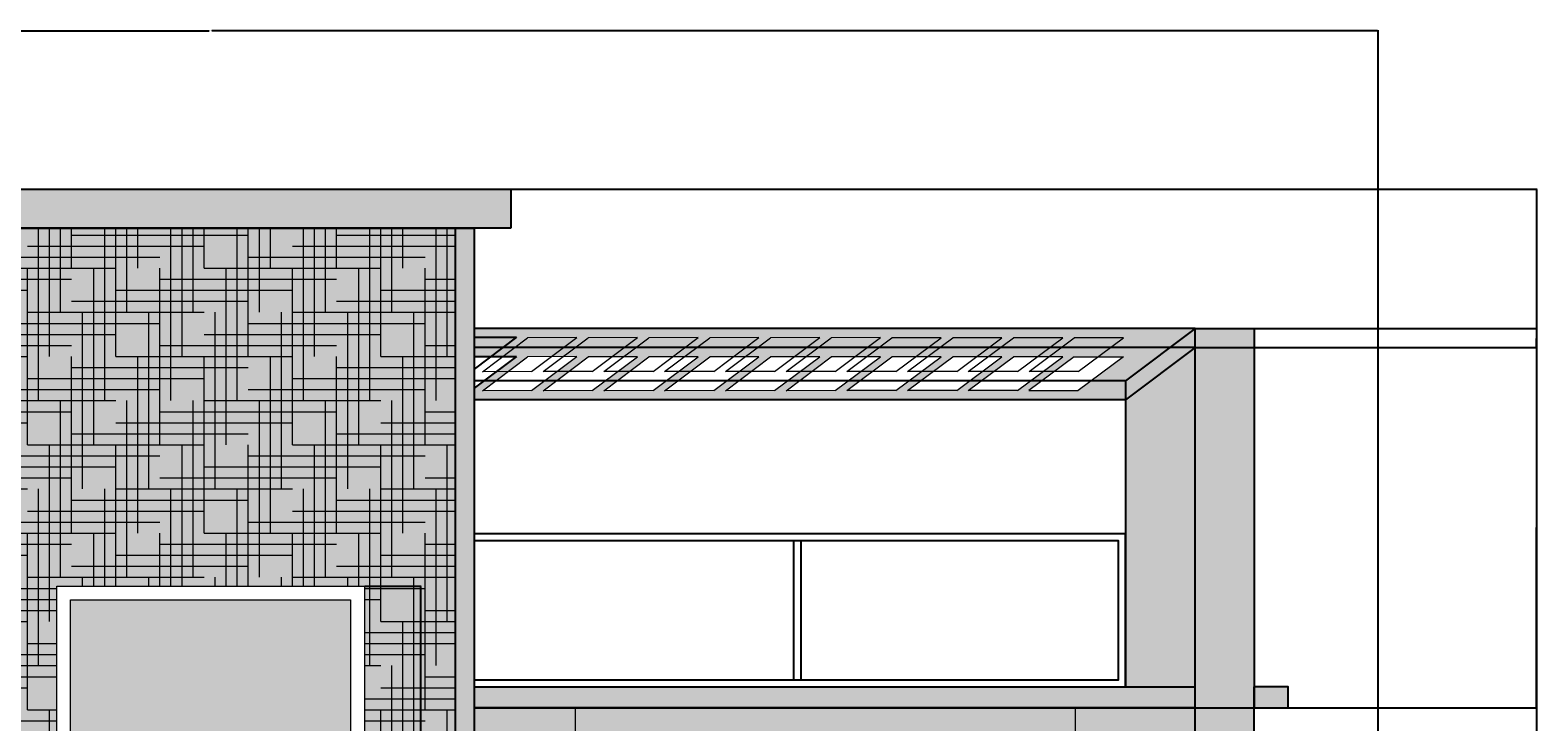
# Model space of a CAD drawing. Units: inches. Extents: x 3024 to 4744, y 1110 to 2100.
# Tile 27 of 29: x 3354 to 3787, y 1902 to 2100. Entities that reach past the tile are written whole.
import ezdxf

# ---------------------------------------------------------------- set-up
doc = ezdxf.new("R2010")
doc.units = ezdxf.units.IN
for name, color, linetype, lineweight in [('A-ANNO-DIMS', 2, 'Continuous', 18), ('A-ELEV', 7, 'Continuous', 25), ('A-ELEV-PATT', 252, 'Continuous', 13), ('A-GLAZ', 4, 'Continuous', 18), ('A-ROOF', 3, 'Continuous', 18)]:
    doc.layers.add(name, color=color, linetype=linetype, lineweight=lineweight)
doc.styles.get("Standard").update_dxf_attribs({"font": 'arial.ttf'})
doc.dimstyles.get("Standard").update_dxf_attribs({"dimtxt": 0.18, "dimasz": 0.18, "dimexe": 0.18, "dimexo": 0.0625, "dimgap": 0.09, "dimtad": 0, "dimtih": 1, "dimtoh": 1, "dimdec": 1, "dimzin": 0, "dimdsep": 46, "dimlunit": 3, "dimtxsty": 'Standard', "dimcen": 0.09, "dimadec": 0, "dimazin": 0, "dimtfac": 1, "dimtdec": 1, "dimtofl": 0, "dimtmove": 0, "dimatfit": 3, "dimfxl": 1, "dimtolj": 1, "dimtzin": 0, "dimarcsym": 0})

# ---------------------------------------------------------------- blocks, each defined once
blk = doc.blocks.new('WIN-BALCONY-A')
for p, q in [((3169.4, 1897.49), (3148.97, 1897.49)), ((3169.4, 1897.49), (3148.97, 1897.49)), ((3169.4, 1897.49), (3292.61, 1897.49)), ((3169.4, 1897.49), (3292.61, 1897.49)), ((3169.4, 1795.04), (3148.97, 1795.04)), ((3169.4, 1795.04), (3148.97, 1795.04)), ((3169.4, 1795.04), (3292.61, 1795.04)), ((3169.4, 1795.04), (3292.61, 1795.04))]:
    blk.add_line(p, q)
for points in [[(3148.97, 1897.49), (3148.97, 1905.61), (3292.61, 1905.61), (3292.61, 1897.49)], [(3148.97, 1897.49), (3148.97, 1905.61), (3292.61, 1905.61), (3292.61, 1897.49)], [(3292.61, 1795.04), (3292.61, 1785.61), (3148.97, 1785.61), (3148.97, 1795.04)], [(3292.61, 1795.04), (3292.61, 1785.61), (3148.97, 1785.61), (3148.97, 1795.04)]]:
    blk.add_lwpolyline(points)
for points in [[(3154.33, 1806.87), (3160.86, 1806.87), (3160.86, 1897.49), (3154.33, 1897.49)], [(3154.33, 1806.87), (3160.86, 1806.87), (3160.86, 1897.49), (3154.33, 1897.49)], [(3272.18, 1795.04), (3169.4, 1795.04), (3169.4, 1897.49), (3272.18, 1897.49)], [(3272.18, 1795.04), (3169.4, 1795.04), (3169.4, 1897.49), (3272.18, 1897.49)], [(3287.25, 1806.87), (3280.72, 1806.87), (3280.72, 1897.49), (3287.25, 1897.49)], [(3287.25, 1806.87), (3280.72, 1806.87), (3280.72, 1897.49), (3287.25, 1897.49)], [(3268.18, 1799.04), (3173.4, 1799.04), (3173.4, 1893.49), (3268.18, 1893.49)], [(3268.18, 1799.04), (3173.4, 1799.04), (3173.4, 1893.49), (3268.18, 1893.49)], [(3220.05, 1893.49), (3221.52, 1893.49), (3221.52, 1799.04), (3220.05, 1799.04)], [(3220.05, 1893.49), (3221.52, 1893.49), (3221.52, 1799.04), (3220.05, 1799.04)], [(3163.53, 1795.04), (3151.66, 1795.04), (3151.66, 1806.87), (3163.53, 1806.87)], [(3163.53, 1795.04), (3151.66, 1795.04), (3151.66, 1806.87), (3163.53, 1806.87)], [(3276.51, 1795.04), (3288.38, 1795.04), (3288.38, 1806.87), (3276.51, 1806.87)], [(3276.51, 1795.04), (3288.38, 1795.04), (3288.38, 1806.87), (3276.51, 1806.87)]]:
    blk.add_lwpolyline(points, close=True)
blk = doc.blocks.new('WIN-STONE-CENTRE')
for points in [[(3361.22, 1940.61), (3449.72, 1940.61), (3449.72, 1833.52), (3361.22, 1833.52)], [(3361.22, 1940.61), (3449.72, 1940.61), (3449.72, 1833.52), (3361.22, 1833.52)], [(3365.22, 1936.61), (3445.72, 1936.61), (3445.72, 1837.52), (3365.22, 1837.52)], [(3365.22, 1936.61), (3445.72, 1936.61), (3445.72, 1837.52), (3365.22, 1837.52)]]:
    blk.add_lwpolyline(points, close=True)
blk = doc.blocks.new('PERGOLA-RAFTER')
for p, q in [((13, 9.73), (0, 0)), ((13, 9.73), (27.14, 9.72)), ((27.14, 9.72), (14.16, 0.01)), ((0, 0), (14.16, 0.01))]:
    blk.add_line(p, q)
blk = doc.blocks.new('*D10')
at = {"layer": 'A-ANNO-DIMS', "color": 0, "lineweight": -2, "transparency": 16777216}
for p, q in [((3449.78, 1940.61), (3465.96, 1940.61)), ((3465.78, 1940.43), (3465.78, 1887.25)), ((3465.78, 1833.7), (3465.78, 1886.88)), ((3449.78, 1833.52), (3465.96, 1833.52))]:
    blk.add_line(p, q, dxfattribs=at)
at = {"layer": 'A-ANNO-DIMS', "color": 0, "transparency": 16777216}
for points in [[(3465.75, 1940.43), (3465.81, 1940.43), (3465.78, 1940.61)], [(3465.75, 1833.7), (3465.81, 1833.7), (3465.78, 1833.52)]]:
    blk.add_solid(points, dxfattribs=at)
at = {"layer": 'Defpoints', "color": 0, "transparency": 16777216}
for p in [(3449.72, 1940.61), (3465.78, 1940.61), (3449.72, 1833.52)]:
    blk.add_point(p, dxfattribs=at)
at = {"layer": 'A-ANNO-DIMS', "color": 0, "transparency": 16777216, "insert": (3465.78, 1887.07), "char_height": 0.18, "attachment_point": 5}
blk.add_mtext('\\A1;STONE WINDOW 107 TYP.', dxfattribs=at)
blk = doc.blocks.new('*D64')
at = {"layer": 'A-ANNO-DIMS', "color": 0, "lineweight": -2, "transparency": 16777216}
for p, q in [((3069.79, 1241.5), (3069.79, 2100.44)), ((3069.97, 2100.26), (3405.08, 2100.26)), ((3740.97, 2100.26), (3405.87, 2100.26)), ((3741.15, 1241.5), (3741.15, 2100.44))]:
    blk.add_line(p, q, dxfattribs=at)
at = {"layer": 'A-ANNO-DIMS', "color": 0, "transparency": 16777216}
for points in [[(3069.97, 2100.29), (3069.97, 2100.23), (3069.79, 2100.26)], [(3740.97, 2100.29), (3740.97, 2100.23), (3741.15, 2100.26)]]:
    blk.add_solid(points, dxfattribs=at)
at = {"layer": 'Defpoints', "color": 0, "transparency": 16777216}
for p in [(3741.15, 2100.26), (3069.79, 1241.43), (3741.15, 1241.43)]:
    blk.add_point(p, dxfattribs=at)
at = {"layer": 'A-ANNO-DIMS', "color": 0, "transparency": 16777216, "insert": (3405.47, 2100.26), "char_height": 0.18, "attachment_point": 5}
blk.add_mtext('\\A1;671.4', dxfattribs=at)
blk = doc.blocks.new('*D75')
at = {"layer": 'A-ANNO-DIMS', "color": 0, "lineweight": -2, "transparency": 16777216}
for p, q in [((3491.89, 2054.76), (3786.83, 2054.76)), ((3786.65, 2054.58), (3786.65, 1605.37)), ((3786.65, 1155.79), (3786.65, 1605)), ((3741.21, 1155.61), (3786.83, 1155.61))]:
    blk.add_line(p, q, dxfattribs=at)
at = {"layer": 'A-ANNO-DIMS', "color": 0, "transparency": 16777216}
for points in [[(3786.62, 2054.58), (3786.68, 2054.58), (3786.65, 2054.76)], [(3786.62, 1155.79), (3786.68, 1155.79), (3786.65, 1155.61)]]:
    blk.add_solid(points, dxfattribs=at)
at = {"layer": 'Defpoints', "color": 0, "transparency": 16777216}
for p in [(3491.83, 2054.76), (3786.65, 2054.76), (3741.15, 1155.61)]:
    blk.add_point(p, dxfattribs=at)
at = {"layer": 'A-ANNO-DIMS', "color": 0, "transparency": 16777216, "insert": (3786.65, 1605.18), "char_height": 0.18, "attachment_point": 5}
blk.add_mtext('\\A1;899.1', dxfattribs=at)
blk = doc.blocks.new('*D80')
at = {"layer": 'A-ANNO-DIMS', "color": 0, "lineweight": -2, "transparency": 16777216}
for p, q in [((3688.62, 2009.17), (3786.83, 2009.17)), ((3786.65, 2008.99), (3786.65, 1957.57)), ((3786.65, 1905.79), (3786.65, 1957.21)), ((3688.62, 1905.61), (3786.83, 1905.61))]:
    blk.add_line(p, q, dxfattribs=at)
at = {"layer": 'A-ANNO-DIMS', "color": 0, "transparency": 16777216}
for points in [[(3786.62, 2008.99), (3786.68, 2008.99), (3786.65, 2009.17)], [(3786.62, 1905.79), (3786.68, 1905.79), (3786.65, 1905.61)]]:
    blk.add_solid(points, dxfattribs=at)
at = {"layer": 'Defpoints', "color": 0, "transparency": 16777216}
for p in [(3688.56, 2009.17), (3786.65, 2009.17), (3688.56, 1905.61)]:
    blk.add_point(p, dxfattribs=at)
at = {"layer": 'A-ANNO-DIMS', "color": 0, "transparency": 16777216, "insert": (3786.65, 1957.39), "char_height": 0.18, "attachment_point": 5}
blk.add_mtext('\\A1;103.56', dxfattribs=at)
blk = doc.blocks.new('*D81')
at = {"layer": 'A-ANNO-DIMS', "color": 0, "lineweight": -2, "transparency": 16777216}
for p, q in [((3705.53, 2014.66), (3786.83, 2014.66)), ((3786.65, 2014.48), (3786.65, 2012.09)), ((3786.65, 2009.35), (3786.65, 2011.73)), ((3688.62, 2009.17), (3786.83, 2009.17))]:
    blk.add_line(p, q, dxfattribs=at)
at = {"layer": 'A-ANNO-DIMS', "color": 0, "transparency": 16777216}
for points in [[(3786.62, 2014.48), (3786.68, 2014.48), (3786.65, 2014.66)], [(3786.62, 2009.35), (3786.68, 2009.35), (3786.65, 2009.17)]]:
    blk.add_solid(points, dxfattribs=at)
at = {"layer": 'Defpoints', "color": 0, "transparency": 16777216}
for p in [(3705.47, 2014.66), (3786.65, 2014.66), (3688.56, 2009.17)]:
    blk.add_point(p, dxfattribs=at)
at = {"layer": 'A-ANNO-DIMS', "color": 0, "transparency": 16777216, "insert": (3786.65, 2011.91), "char_height": 0.18, "attachment_point": 5}
blk.add_mtext('\\A1;5.49', dxfattribs=at)

msp = doc.modelspace()

# ---------------------------------------------------------------- hatches: boundary and pattern name
at = {"layer": 'A-ELEV-PATT'}
h = msp.add_hatch(color=256, dxfattribs=at)
h.dxf.hatch_style = 1
h.paths.add_polyline_path([(3491.8271, 2054.7584), (3320.5658, 2054.7584), (3320.5658, 2043.5286), (3491.8271, 2043.5286)])
h.paths.add_polyline_path([(3292.6051, 1905.6112), (3148.9694, 1905.6112), (3148.9694, 1897.4879), (3169.3964, 1897.4879), (3292.6051, 1897.4879)])
h.paths.add_polyline_path([(3292.6051, 1795.0431), (3169.3964, 1795.0431), (3148.9694, 1795.0431), (3148.9694, 1785.6112), (3292.6051, 1785.6112)])
h.paths.add_polyline_path([(3292.6051, 1779.6112), (3148.9694, 1779.6112), (3148.9694, 1771.4879), (3169.3964, 1771.4879), (3292.6051, 1771.4879)])
h.paths.add_polyline_path([(3292.6051, 1669.0431), (3169.3964, 1669.0431), (3148.9694, 1669.0431), (3148.9694, 1659.6112), (3292.6051, 1659.6112)])
h.paths.add_polyline_path([(3292.6051, 1653.6112), (3148.9694, 1653.6112), (3148.9694, 1645.4879), (3169.3964, 1645.4879), (3292.6051, 1645.4879)])
h.paths.add_polyline_path([(3292.6051, 1543.0431), (3169.3964, 1543.0431), (3148.9694, 1543.0431), (3148.9694, 1533.6112), (3292.6051, 1533.6112)])
h.paths.add_polyline_path([(3292.6051, 1527.6112), (3148.9694, 1527.6112), (3148.9694, 1519.4879), (3169.3964, 1519.4879), (3292.6051, 1519.4879)])
h.paths.add_polyline_path([(3292.6051, 1401.6112), (3148.9694, 1401.6112), (3148.9694, 1393.4879), (3169.3964, 1393.4879), (3292.6051, 1393.4879)])
h.paths.add_polyline_path([(3292.6051, 1417.0431), (3169.3964, 1417.0431), (3148.9694, 1417.0431), (3148.9694, 1407.6112), (3292.6051, 1407.6112)])
h.paths.add_polyline_path([(3292.6051, 1291.0431), (3169.3964, 1291.0431), (3148.9694, 1291.0431), (3148.9694, 1281.6112), (3292.6051, 1281.6112)])
h.paths.add_polyline_path([(3654.037, 1165.0431), (3530.8283, 1165.0431), (3510.4013, 1165.0431), (3510.4013, 1155.6112), (3654.037, 1155.6112)])
h.paths.add_polyline_path([(3654.037, 1275.6112), (3510.4013, 1275.6112), (3510.4013, 1267.4879), (3530.8283, 1267.4879), (3654.037, 1267.4879)])
h.paths.add_polyline_path([(3654.037, 1291.0431), (3530.8283, 1291.0431), (3510.4013, 1291.0431), (3510.4013, 1281.6112), (3654.037, 1281.6112)])
h.paths.add_polyline_path([(3654.037, 1417.0431), (3530.8283, 1417.0431), (3510.4013, 1417.0431), (3510.4013, 1407.6112), (3654.037, 1407.6112)])
h.paths.add_polyline_path([(3654.037, 1401.6112), (3510.4013, 1401.6112), (3510.4013, 1393.4879), (3530.8283, 1393.4879), (3654.037, 1393.4879)])
h.paths.add_polyline_path([(3654.037, 1543.0431), (3530.8283, 1543.0431), (3510.4013, 1543.0431), (3510.4013, 1533.6112), (3654.037, 1533.6112)])
h.paths.add_polyline_path([(3654.037, 1527.6112), (3510.4013, 1527.6112), (3510.4013, 1519.4879), (3530.8283, 1519.4879), (3654.037, 1519.4879)])
h.paths.add_polyline_path([(3654.037, 1653.6112), (3510.4013, 1653.6112), (3510.4013, 1645.4879), (3530.8283, 1645.4879), (3654.037, 1645.4879)])
h.paths.add_polyline_path([(3654.037, 1669.0431), (3530.8283, 1669.0431), (3510.4013, 1669.0431), (3510.4013, 1659.6112), (3654.037, 1659.6112)])
h.paths.add_polyline_path([(3654.037, 1779.6112), (3510.4013, 1779.6112), (3510.4013, 1771.4879), (3530.8283, 1771.4879), (3654.037, 1771.4879)])
h.paths.add_polyline_path([(3654.037, 1795.0431), (3530.8283, 1795.0431), (3510.4013, 1795.0431), (3510.4013, 1785.6112), (3654.037, 1785.6112)])
h.paths.add_polyline_path([(3654.037, 1905.6112), (3510.4013, 1905.6112), (3510.4013, 1897.4879), (3530.8283, 1897.4879), (3654.037, 1897.4879)])
h = msp.add_hatch(color=256, dxfattribs=at)
h.dxf.hatch_style = 1
h.paths.add_polyline_path([(3335.1044, 2043.5286), (3329.7033, 2043.5286), (3329.7033, 1155.6112), (3335.1044, 1155.6112)])
h.paths.add_polyline_path([(3481.2411, 2043.5286), (3335.1044, 2043.5286), (3335.1044, 1155.6112), (3481.2411, 1155.6112)])
h.paths.add_polyline_path([(3449.7202, 1329.5246), (3361.2242, 1329.5246), (3361.2242, 1436.6064), (3449.7202, 1436.6064)], flags=16)
h.paths.add_polyline_path([(3445.7202, 1333.5246), (3365.2242, 1333.5246), (3365.2242, 1432.6064), (3445.7202, 1432.6064)], flags=0)
h.paths.add_polyline_path([(3449.7202, 1455.5246), (3361.2242, 1455.5246), (3361.2242, 1562.6064), (3449.7202, 1562.6064)], flags=16)
h.paths.add_polyline_path([(3445.7202, 1459.5246), (3365.2242, 1459.5246), (3365.2242, 1558.6064), (3445.7202, 1558.6064)], flags=0)
h.paths.add_polyline_path([(3449.7202, 1581.5246), (3361.2242, 1581.5246), (3361.2242, 1688.6064), (3449.7202, 1688.6064)], flags=16)
h.paths.add_polyline_path([(3445.7202, 1585.5246), (3365.2242, 1585.5246), (3365.2242, 1684.6064), (3445.7202, 1684.6064)], flags=0)
h.paths.add_polyline_path([(3449.7202, 1707.5246), (3361.2242, 1707.5246), (3361.2242, 1814.6064), (3449.7202, 1814.6064)], flags=16)
h.paths.add_polyline_path([(3445.7202, 1711.5246), (3365.2242, 1711.5246), (3365.2242, 1810.6064), (3445.7202, 1810.6064)], flags=0)
h.paths.add_polyline_path([(3449.7202, 1833.5246), (3361.2242, 1833.5246), (3361.2242, 1940.6064), (3449.7202, 1940.6064)], flags=16)
h.paths.add_polyline_path([(3445.7202, 1837.5246), (3365.2242, 1837.5246), (3365.2242, 1936.6064), (3445.7202, 1936.6064)], flags=0)
h = msp.add_hatch(color=256, dxfattribs=at)
h.dxf.hatch_style = 1
h.paths.add_polyline_path([(3475.84, 2043.5286), (3335.1044, 2043.5286), (3335.1044, 1155.6112), (3475.84, 1155.6112)])
h.paths.add_polyline_path([(3449.7202, 1940.6064), (3449.7202, 1833.5246), (3361.2242, 1833.5246), (3361.2242, 1940.6064)], flags=16)
h.paths.add_polyline_path([(3445.7202, 1936.6064), (3445.7202, 1837.5246), (3365.2242, 1837.5246), (3365.2242, 1936.6064)], flags=0)
h.paths.add_polyline_path([(3449.7202, 1814.6064), (3449.7202, 1707.5246), (3361.2242, 1707.5246), (3361.2242, 1814.6064)], flags=16)
h.paths.add_polyline_path([(3445.7202, 1810.6064), (3445.7202, 1711.5246), (3365.2242, 1711.5246), (3365.2242, 1810.6064)], flags=0)
h.paths.add_polyline_path([(3449.7202, 1688.6064), (3449.7202, 1581.5246), (3361.2242, 1581.5246), (3361.2242, 1688.6064)], flags=16)
h.paths.add_polyline_path([(3445.7202, 1684.6064), (3445.7202, 1585.5246), (3365.2242, 1585.5246), (3365.2242, 1684.6064)], flags=0)
h.paths.add_polyline_path([(3449.7202, 1562.6064), (3449.7202, 1455.5246), (3361.2242, 1455.5246), (3361.2242, 1562.6064)], flags=16)
h.paths.add_polyline_path([(3445.7202, 1558.6064), (3445.7202, 1459.5246), (3365.2242, 1459.5246), (3365.2242, 1558.6064)], flags=0)
h.paths.add_polyline_path([(3449.7202, 1436.6064), (3449.7202, 1329.5246), (3361.2242, 1329.5246), (3361.2242, 1436.6064)], flags=16)
h.paths.add_polyline_path([(3445.7202, 1432.6064), (3445.7202, 1333.5246), (3365.2242, 1333.5246), (3365.2242, 1432.6064)], flags=0)
h = msp.add_hatch(dxfattribs=at)
h.set_pattern_fill('HOUND', color=256, scale=2)
h.paths.add_polyline_path([(3475.84, 2043.5286), (3335.1044, 2043.5286), (3335.1044, 1155.6112), (3475.84, 1155.6112)])
h.paths.add_polyline_path([(3449.7202, 1940.6064), (3449.7202, 1833.5246), (3361.2242, 1833.5246), (3361.2242, 1940.6064)], flags=16)
h.paths.add_polyline_path([(3445.7202, 1936.6064), (3445.7202, 1837.5246), (3365.2242, 1837.5246), (3365.2242, 1936.6064)], flags=0)
h.paths.add_polyline_path([(3449.7202, 1814.6064), (3449.7202, 1707.5246), (3361.2242, 1707.5246), (3361.2242, 1814.6064)], flags=16)
h.paths.add_polyline_path([(3445.7202, 1810.6064), (3445.7202, 1711.5246), (3365.2242, 1711.5246), (3365.2242, 1810.6064)], flags=0)
h.paths.add_polyline_path([(3449.7202, 1688.6064), (3449.7202, 1581.5246), (3361.2242, 1581.5246), (3361.2242, 1688.6064)], flags=16)
h.paths.add_polyline_path([(3445.7202, 1684.6064), (3445.7202, 1585.5246), (3365.2242, 1585.5246), (3365.2242, 1684.6064)], flags=0)
h.paths.add_polyline_path([(3449.7202, 1562.6064), (3449.7202, 1455.5246), (3361.2242, 1455.5246), (3361.2242, 1562.6064)], flags=16)
h.paths.add_polyline_path([(3445.7202, 1558.6064), (3445.7202, 1459.5246), (3365.2242, 1459.5246), (3365.2242, 1558.6064)], flags=0)
h.paths.add_polyline_path([(3449.7202, 1436.6064), (3449.7202, 1329.5246), (3361.2242, 1329.5246), (3361.2242, 1436.6064)], flags=16)
h.paths.add_polyline_path([(3445.7202, 1432.6064), (3445.7202, 1333.5246), (3365.2242, 1333.5246), (3365.2242, 1432.6064)], flags=0)
h = msp.add_hatch(color=256, dxfattribs=at)
h.dxf.hatch_style = 1
h.paths.add_polyline_path([(3582.956, 2019.4879), (3581.4824, 2019.4879), (3581.4824, 1925.0431), (3582.956, 1925.0431)], flags=0)
h.paths.add_polyline_path([(3582.956, 2019.4879), (3582.956, 1925.0431), (3581.4824, 1925.0431), (3581.4824, 2019.4879)], flags=0)
h.paths.add_polyline_path([(3582.956, 1893.4879), (3581.4824, 1893.4879), (3581.4824, 1799.0431), (3582.956, 1799.0431)])
h = msp.add_hatch(color=256, dxfattribs=at)
h.dxf.hatch_style = 1
h.paths.add_polyline_path([(3705.4722, 2014.6567), (3688.5588, 2014.6567), (3481.2411, 2014.6567), (3481.2411, 2009.1664), (3688.5588, 2009.1664), (3688.5588, 1155.6112), (3705.4722, 1155.6112), (3705.4722, 1911.6112)])
h = msp.add_hatch(color=256, dxfattribs=at)
h.dxf.hatch_style = 1
h.paths.add_polyline_path([(3688.5588, 2009.1664), (3481.2411, 2009.1664), (3481.2411, 2006.6317), (3493.4114, 2006.6233), (3481.2411, 1997.5141), (3481.2411, 1994.1371), (3668.4791, 1994.1371)])
h.paths.add_polyline_path([(3515.0719, 1996.695), (3500.9072, 1996.6853), (3514.1658, 2006.6091), (3528.3045, 2006.5994)], flags=16)
h.paths.add_polyline_path([(3518.3858, 1996.6973), (3531.6123, 2006.5971), (3545.751, 2006.5874), (3532.5505, 1996.707)], flags=16)
h.paths.add_polyline_path([(3497.5933, 1996.683), (3483.4286, 1996.6733), (3496.7192, 2006.6211), (3510.8579, 2006.6113)], flags=16)
h.paths.add_polyline_path([(3535.8644, 1996.7093), (3549.0589, 2006.5851), (3563.1976, 2006.5754), (3550.0291, 1996.719)], flags=16)
h.paths.add_polyline_path([(3553.343, 1996.7213), (3566.5055, 2006.5731), (3580.6442, 2006.5634), (3567.5077, 1996.731)], flags=16)
h.paths.add_polyline_path([(3570.8217, 1996.7333), (3583.952, 2006.5611), (3598.0907, 2006.5514), (3584.9863, 1996.743)], flags=16)
h.paths.add_polyline_path([(3588.3003, 1996.7453), (3601.3986, 2006.5492), (3615.5373, 2006.5395), (3602.465, 1996.755)], flags=16)
h.paths.add_polyline_path([(3605.7789, 1996.7573), (3618.8451, 2006.5372), (3632.9839, 2006.5275), (3619.9436, 1996.767)], flags=16)
h.paths.add_polyline_path([(3623.2575, 1996.7693), (3636.2917, 2006.5252), (3650.4304, 2006.5155), (3637.4222, 1996.779)], flags=16)
h.paths.add_polyline_path([(3640.7361, 1996.7813), (3653.7383, 2006.5132), (3667.877, 2006.5035), (3654.9008, 1996.7911)], flags=16)
h.paths.add_polyline_path([(3688.5588, 2009.1664), (3668.4791, 1994.1371), (3668.4791, 1911.6112), (3688.5588, 1911.6112)])
h = msp.add_hatch(color=256, dxfattribs=at)
h.dxf.hatch_style = 1
h.paths.add_polyline_path([(3445.7202, 1936.6064), (3365.2242, 1936.6064), (3365.2242, 1837.5246), (3445.7202, 1837.5246)])
h.paths.add_polyline_path([(3445.7202, 1810.6064), (3365.2242, 1810.6064), (3365.2242, 1711.5246), (3445.7202, 1711.5246)])
h.paths.add_polyline_path([(3445.7202, 1684.6064), (3365.2242, 1684.6064), (3365.2242, 1585.5246), (3445.7202, 1585.5246)])
h.paths.add_polyline_path([(3445.7202, 1558.6064), (3365.2242, 1558.6064), (3365.2242, 1459.5246), (3445.7202, 1459.5246)])
h.paths.add_polyline_path([(3445.7202, 1432.6064), (3365.2242, 1432.6064), (3365.2242, 1333.5246), (3445.7202, 1333.5246)])
h = msp.add_hatch(color=256, dxfattribs=at)
h.dxf.hatch_style = 1
h.paths.add_polyline_path([(3329.7033, 1407.6112), (3105.4722, 1407.6112), (3105.4722, 1401.6112), (3329.7033, 1401.6112)])
h.paths.add_polyline_path([(3329.7033, 1281.6112), (3105.4722, 1281.6112), (3105.4722, 1275.6112), (3112.3838, 1275.6112), (3329.7033, 1275.6112)])
h.paths.add_polyline_path([(3329.7033, 1533.6112), (3105.4722, 1533.6112), (3105.4722, 1527.6112), (3329.7033, 1527.6112)])
h.paths.add_polyline_path([(3329.7033, 1659.6112), (3105.4722, 1659.6112), (3105.4722, 1653.6112), (3329.7033, 1653.6112)])
h.paths.add_polyline_path([(3329.7033, 1785.6112), (3105.4722, 1785.6112), (3105.4722, 1779.6112), (3329.7033, 1779.6112)])
h.paths.add_polyline_path([(3329.7033, 1911.6112), (3105.4722, 1911.6112), (3095.7158, 1911.6112), (3095.7158, 1905.6112), (3329.7033, 1905.6112)])
h.paths.add_polyline_path([(3715.2286, 1911.6112), (3705.4722, 1911.6112), (3705.4722, 1905.6112), (3715.2286, 1905.6112)])
h.paths.add_polyline_path([(3688.5588, 1911.6112), (3481.2411, 1911.6112), (3481.2411, 1905.6112), (3688.5588, 1905.6112)])
h = msp.add_hatch(color=256, dxfattribs=at)
h.dxf.hatch_style = 1
h.paths.add_polyline_path([(3154.3287, 1897.4879), (3148.9694, 1897.4879), (3148.9694, 1905.6112), (3105.4722, 1905.6112), (3105.4722, 1785.6112), (3148.9694, 1785.6112), (3148.9694, 1795.0431), (3151.6604, 1795.0431), (3151.6604, 1806.8674), (3154.3287, 1806.8674)])
h.paths.add_polyline_path([(3329.7033, 1905.6112), (3292.6051, 1905.6112), (3292.6051, 1897.4879), (3287.2458, 1897.4879), (3287.2458, 1806.8674), (3288.3759, 1806.8674), (3288.3759, 1795.0431), (3292.6051, 1795.0431), (3292.6051, 1785.6112), (3329.7033, 1785.6112)])
h.paths.add_polyline_path([(3154.3287, 1771.4879), (3148.9694, 1771.4879), (3148.9694, 1779.6112), (3105.4722, 1779.6112), (3105.4722, 1659.6112), (3148.9694, 1659.6112), (3148.9694, 1669.0431), (3151.6604, 1669.0431), (3151.6604, 1680.8674), (3154.3287, 1680.8674)])
h.paths.add_polyline_path([(3329.7033, 1779.6112), (3292.6051, 1779.6112), (3292.6051, 1771.4879), (3287.2458, 1771.4879), (3287.2458, 1680.8674), (3288.3759, 1680.8674), (3288.3759, 1669.0431), (3292.6051, 1669.0431), (3292.6051, 1659.6112), (3329.7033, 1659.6112)])
h.paths.add_polyline_path([(3154.3287, 1645.4879), (3148.9694, 1645.4879), (3148.9694, 1653.6112), (3105.4722, 1653.6112), (3105.4722, 1533.6112), (3148.9694, 1533.6112), (3148.9694, 1543.0431), (3151.6604, 1543.0431), (3151.6604, 1554.8674), (3154.3287, 1554.8674)])
h.paths.add_polyline_path([(3329.7033, 1653.6112), (3292.6051, 1653.6112), (3292.6051, 1645.4879), (3287.2458, 1645.4879), (3287.2458, 1554.8674), (3288.3759, 1554.8674), (3288.3759, 1543.0431), (3292.6051, 1543.0431), (3292.6051, 1533.6112), (3329.7033, 1533.6112)])
h.paths.add_polyline_path([(3329.7033, 1527.6112), (3292.6051, 1527.6112), (3292.6051, 1519.4879), (3287.2458, 1519.4879), (3287.2458, 1428.8674), (3288.3759, 1428.8674), (3288.3759, 1417.0431), (3292.6051, 1417.0431), (3292.6051, 1407.6112), (3329.7033, 1407.6112)])
h.paths.add_polyline_path([(3329.7033, 1401.6112), (3292.6051, 1401.6112), (3292.6051, 1393.4879), (3287.2458, 1393.4879), (3287.2458, 1302.8674), (3288.3759, 1302.8674), (3288.3759, 1291.0431), (3292.6051, 1291.0431), (3292.6051, 1281.6112), (3329.7033, 1281.6112)])
h.paths.add_polyline_path([(3154.3287, 1393.4879), (3148.9694, 1393.4879), (3148.9694, 1401.6112), (3105.4722, 1401.6112), (3105.4722, 1281.6112), (3148.9694, 1281.6112), (3148.9694, 1291.0431), (3151.6604, 1291.0431), (3151.6604, 1302.8674), (3154.3287, 1302.8674)])
h.paths.add_polyline_path([(3154.3287, 1519.4879), (3148.9694, 1519.4879), (3148.9694, 1527.6112), (3105.4722, 1527.6112), (3105.4722, 1407.6112), (3148.9694, 1407.6112), (3148.9694, 1417.0431), (3151.6604, 1417.0431), (3151.6604, 1428.8674), (3154.3287, 1428.8674)])
h.paths.add_polyline_path([(3515.7606, 1897.4879), (3510.4013, 1897.4879), (3510.4013, 1905.6112), (3481.2411, 1905.6112), (3481.2411, 1785.6112), (3510.4013, 1785.6112), (3510.4013, 1795.0431), (3513.0923, 1795.0431), (3513.0923, 1806.8674), (3515.7606, 1806.8674)])
h.paths.add_polyline_path([(3688.5588, 1905.6112), (3654.037, 1905.6112), (3654.037, 1897.4879), (3648.6777, 1897.4879), (3648.6777, 1806.8674), (3649.8078, 1806.8674), (3649.8078, 1795.0431), (3654.037, 1795.0431), (3654.037, 1785.6112), (3688.5588, 1785.6112)])
h.paths.add_polyline_path([(3515.7606, 1771.4879), (3510.4013, 1771.4879), (3510.4013, 1779.6112), (3481.2411, 1779.6112), (3481.2411, 1659.6112), (3510.4013, 1659.6112), (3510.4013, 1669.0431), (3513.0923, 1669.0431), (3513.0923, 1680.8674), (3515.7606, 1680.8674)])
h.paths.add_polyline_path([(3688.5588, 1779.6112), (3654.037, 1779.6112), (3654.037, 1771.4879), (3648.6777, 1771.4879), (3648.6777, 1680.8674), (3649.8078, 1680.8674), (3649.8078, 1669.0431), (3654.037, 1669.0431), (3654.037, 1659.6112), (3688.5588, 1659.6112)])
h.paths.add_polyline_path([(3515.7606, 1645.4879), (3510.4013, 1645.4879), (3510.4013, 1653.6112), (3481.2411, 1653.6112), (3481.2411, 1533.6112), (3510.4013, 1533.6112), (3510.4013, 1543.0431), (3513.0923, 1543.0431), (3513.0923, 1554.8674), (3515.7606, 1554.8674)])
h.paths.add_polyline_path([(3688.5588, 1653.6112), (3654.037, 1653.6112), (3654.037, 1645.4879), (3648.6777, 1645.4879), (3648.6777, 1554.8674), (3649.8078, 1554.8674), (3649.8078, 1543.0431), (3654.037, 1543.0431), (3654.037, 1533.6112), (3688.5588, 1533.6112)])
h.paths.add_polyline_path([(3515.7606, 1519.4879), (3510.4013, 1519.4879), (3510.4013, 1527.6112), (3481.2411, 1527.6112), (3481.2411, 1407.6112), (3510.4013, 1407.6112), (3510.4013, 1417.0431), (3513.0923, 1417.0431), (3513.0923, 1428.8674), (3515.7606, 1428.8674)])
h.paths.add_polyline_path([(3688.5588, 1527.6112), (3654.037, 1527.6112), (3654.037, 1519.4879), (3648.6777, 1519.4879), (3648.6777, 1428.8674), (3649.8078, 1428.8674), (3649.8078, 1417.0431), (3654.037, 1417.0431), (3654.037, 1407.6112), (3688.5588, 1407.6112)])
h.paths.add_polyline_path([(3515.7606, 1393.4879), (3510.4013, 1393.4879), (3510.4013, 1401.6112), (3481.2411, 1401.6112), (3481.2411, 1281.6112), (3510.4013, 1281.6112), (3510.4013, 1291.0431), (3513.0923, 1291.0431), (3513.0923, 1302.8674), (3515.7606, 1302.8674)])
h.paths.add_polyline_path([(3688.5588, 1401.6112), (3654.037, 1401.6112), (3654.037, 1393.4879), (3648.6777, 1393.4879), (3648.6777, 1302.8674), (3649.8078, 1302.8674), (3649.8078, 1291.0431), (3654.037, 1291.0431), (3654.037, 1281.6112), (3688.5588, 1281.6112)])
h.paths.add_polyline_path([(3515.7606, 1267.4879), (3510.4013, 1267.4879), (3510.4013, 1275.6112), (3481.2411, 1275.6112), (3481.2411, 1155.6112), (3510.4013, 1155.6112), (3510.4013, 1165.0431), (3513.0923, 1165.0431), (3513.0923, 1176.8674), (3515.7606, 1176.8674)])
h.paths.add_polyline_path([(3688.5588, 1275.6112), (3654.037, 1275.6112), (3654.037, 1267.4879), (3648.6777, 1267.4879), (3648.6777, 1176.8674), (3649.8078, 1176.8674), (3649.8078, 1165.0431), (3654.037, 1165.0431), (3654.037, 1155.6112), (3688.5588, 1155.6112)])
h.paths.add_polyline_path([(3112.3838, 1275.6112), (3105.4722, 1275.6112), (3105.4722, 1171.0239), (3112.3838, 1171.0239)])

# ---------------------------------------------------------------- linework, layer by layer
at = {"layer": 'A-ELEV'}
for p, q in [((3688.5588, 2014.6567), (3481.2411, 2014.6567)), ((3688.5588, 2014.6567), (3481.2411, 2014.6567)), ((3481.2411, 2012.122), (3493.4114, 2012.1136)), ((3493.4114, 2012.1136), (3481.2411, 2003.0044)), ((3688.5588, 2014.6567), (3668.4791, 1999.6274)), ((3688.5588, 2009.1664), (3481.2411, 2009.1664)), ((3688.5588, 2009.1664), (3668.4791, 1994.1371)), ((3481.2411, 2006.6317), (3493.4114, 2006.6233)), ((3493.4114, 2006.6233), (3481.2411, 1997.5141)), ((3668.4791, 1999.6274), (3481.2411, 1999.6274)), ((3668.4791, 1999.6274), (3668.4791, 1911.6112)), ((3668.4791, 1994.1371), (3481.2411, 1994.1371)), ((3668.4791, 1994.1371), (3668.4791, 1911.6112)), ((3481.2411, 1911.6112), (3688.5588, 1911.6112)), ((3481.2411, 1911.6112), (3688.5588, 1911.6112)), ((3705.4722, 1155.6112), (3705.4722, 1911.6112)), ((3705.4722, 1155.6112), (3705.4722, 1911.6112)), ((3688.5588, 1905.6112), (3481.2411, 1905.6112)), ((3688.5588, 1905.6112), (3481.2411, 1905.6112))]:
    msp.add_line(p, q, dxfattribs=at)
for points in [[(3491.8271, 2043.5286), (3320.5658, 2043.5286), (3320.5658, 2054.7584), (3491.8271, 2054.7584)], [(3491.8271, 2043.5286), (3320.5658, 2043.5286), (3320.5658, 2054.7584), (3491.8271, 2054.7584)], [(3481.2411, 1155.6112), (3329.7033, 1155.6112), (3329.7033, 2043.5286), (3481.2411, 2043.5286)], [(3481.2411, 1155.6112), (3329.7033, 1155.6112), (3329.7033, 2043.5286), (3481.2411, 2043.5286)], [(3475.84, 2043.5286), (3481.2411, 2043.5286), (3481.2411, 1155.6112), (3475.84, 1155.6112)], [(3475.84, 2043.5286), (3481.2411, 2043.5286), (3481.2411, 1155.6112), (3475.84, 1155.6112)], [(3475.84, 2043.5286), (3481.2411, 2043.5286), (3481.2411, 1155.6112), (3475.84, 1155.6112)]]:
    msp.add_lwpolyline(points, close=True, dxfattribs=at)
for points in [[(3688.5588, 2014.6567), (3705.4722, 2014.6567), (3705.4722, 1905.6112)], [(3705.4722, 1155.6112), (3688.5588, 1155.6112), (3688.5588, 2014.6567), (3705.4722, 2014.6567), (3705.4722, 1905.6112)], [(3705.4722, 1155.6112), (3688.5588, 1155.6112), (3688.5588, 2009.1664)], [(3481.2411, 1911.6112), (3668.4791, 1911.6112), (3668.4791, 1955.6193), (3481.2411, 1955.6193)], [(3481.2411, 1911.6112), (3668.4791, 1911.6112), (3668.4791, 1955.6193), (3481.2411, 1955.6193)], [(3481.2411, 1913.6112), (3666.4791, 1913.6112), (3666.4791, 1953.6193), (3481.2411, 1953.6193)], [(3481.2411, 1913.6112), (3666.4791, 1913.6112), (3666.4791, 1953.6193), (3481.2411, 1953.6193)], [(3573.1321, 1913.6112), (3573.1321, 1953.6193)], [(3573.1321, 1913.6112), (3573.1321, 1953.6193)], [(3575.1321, 1953.6193), (3575.1321, 1913.6112)], [(3575.1321, 1953.6193), (3575.1321, 1913.6112)], [(3481.2411, 1911.6112), (3481.2411, 1905.6112), (3688.5588, 1905.6112)], [(3481.2411, 1911.6112), (3481.2411, 1905.6112), (3688.5588, 1905.6112)], [(3705.4722, 1905.6112), (3715.2286, 1905.6112), (3715.2286, 1911.6112), (3705.4722, 1911.6112)], [(3705.4722, 1905.6112), (3715.2286, 1905.6112), (3715.2286, 1911.6112), (3705.4722, 1911.6112)]]:
    msp.add_lwpolyline(points, dxfattribs=at)

# ---------------------------------------------------------------- block references
at = {"layer": 'A-GLAZ'}
for name, p in [('WIN-STONE-CENTRE', (0, 0)), ('WIN-BALCONY-A', (361.4319, 0))]:
    msp.add_blockref(name, p, dxfattribs=at)
at = {"layer": 'A-ROOF'}
for p, rotation in [((3510.7106, 2012.0486), 180.1893702113597), ((3528.1752, 2012.0432), 180.1664655150032), ((3545.6397, 2012.0377), 180.1435004991811), ((3563.1043, 2012.0323), 180.1204749327245), ((3580.5688, 2012.0268), 180.0973885832933), ((3598.0334, 2012.0214), 180.0742412174357), ((3615.498, 2012.0159), 180.0510326004891), ((3632.9625, 2012.0104), 180.0277624966956), ((3650.4271, 2012.0049), 180.0044306689292), ((3667.8917, 2011.9993), 179.9810368794876), ((3510.7106, 2006.5583), 180.1893702113597), ((3528.1752, 2006.5529), 180.1664655149988), ((3545.6397, 2006.5475), 180.1435004991862), ((3563.1043, 2006.542), 180.1204749327245), ((3580.5688, 2006.5366), 180.097388583297), ((3598.0334, 2006.5311), 180.0742412174357), ((3615.498, 2006.5256), 180.0510326004891), ((3632.9625, 2006.5201), 180.0277624966956), ((3650.4271, 2006.5146), 180.0044306689292)]:
    msp.add_blockref('PERGOLA-RAFTER', p, dxfattribs=dict(at, rotation=rotation))
msp.add_blockref('PERGOLA-RAFTER', (3640.736, 1996.781), dxfattribs=at)

# ---------------------------------------------------------------- dimensions: what is measured, and where the dimension line sits
at = {"layer": 'A-ANNO-DIMS'}
dim = msp.add_linear_dim(base=(3741.1507, 2100.2584), p1=(3069.7937, 1241.4341), p2=(3741.1507, 1241.4341), dimstyle='Standard', override={"dimdec": 1, "dimlfac": 1, "dimrnd": 0, "dimzin": 0, "dimdsep": 46, "dimlunit": 2}, dxfattribs=at)
dim.commit()
dim.dimension.update_dxf_attribs({"geometry": '*D64', "text_midpoint": (3405.4722, 2100.2584)})
for base, p1, p2, override, picture, middle in [((3786.6507, 2054.7584), (3741.1507, 1155.6112), (3491.8271, 2054.7584), {"dimdec": 1, "dimlfac": 1, "dimrnd": 0, "dimzin": 0, "dimdsep": 46, "dimlunit": 2}, '*D75', (3786.6507, 1605.1848)), ((3786.6507, 2014.6567), (3688.5588, 2009.1664), (3705.4722, 2014.6567), {"dimdec": 2, "dimlfac": 1, "dimrnd": 0, "dimzin": 0, "dimdsep": 46, "dimlunit": 2}, '*D81', (3786.6507, 2011.9115)), ((3786.6507, 2009.1664), (3688.5588, 1905.6112), (3688.5588, 2009.1664), {"dimdec": 2, "dimlfac": 1, "dimrnd": 0, "dimzin": 0, "dimdsep": 46, "dimlunit": 2}, '*D80', (3786.6507, 1957.3888))]:
    dim = msp.add_linear_dim(base=base, p1=p1, p2=p2, angle=90, dimstyle='Standard', override=override, dxfattribs=at)
    dim.commit()
    dim.dimension.update_dxf_attribs({"geometry": picture, "text_midpoint": middle})
dim = msp.add_linear_dim(base=(3465.7825, 1940.6064), p1=(3449.7202, 1833.5246), p2=(3449.7202, 1940.6064), angle=90, text='STONE WINDOW <> TYP.', dimstyle='Standard', override={"dimdec": 0, "dimrnd": 0, "dimzin": 0, "dimlunit": 2}, dxfattribs=at)
dim.commit()
dim.dimension.update_dxf_attribs({"geometry": '*D10', "text_midpoint": (3465.7825, 1887.0655)})

doc.saveas('drawing.dxf')
